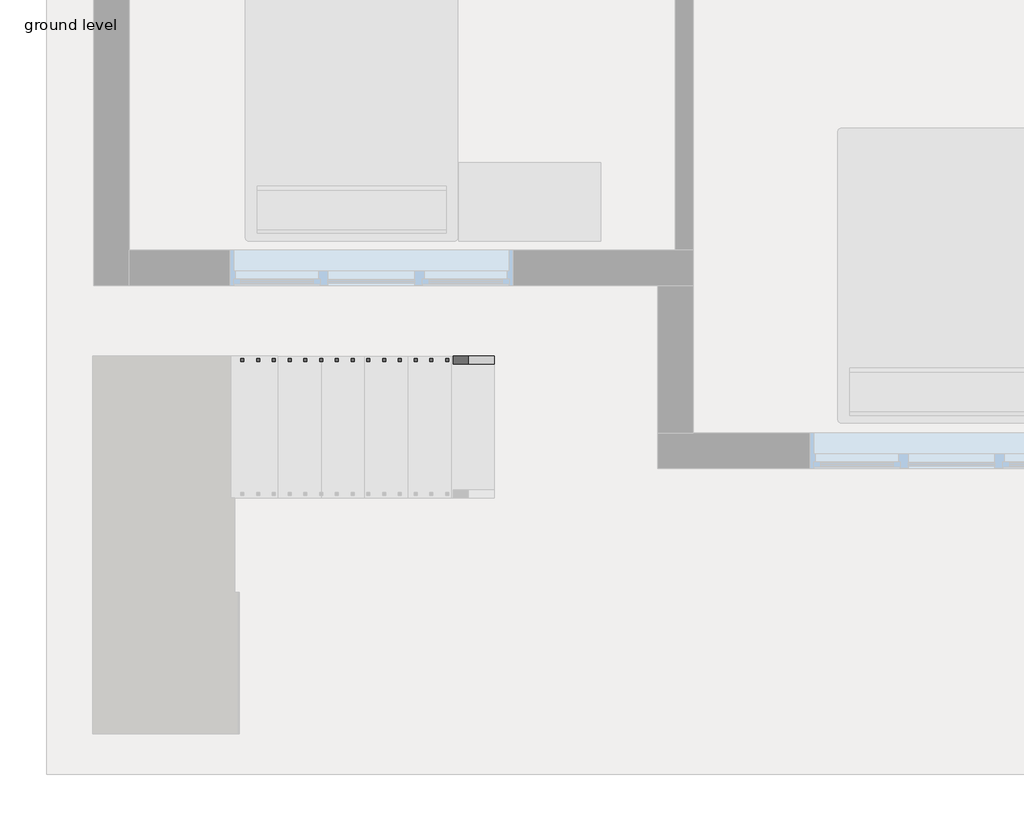
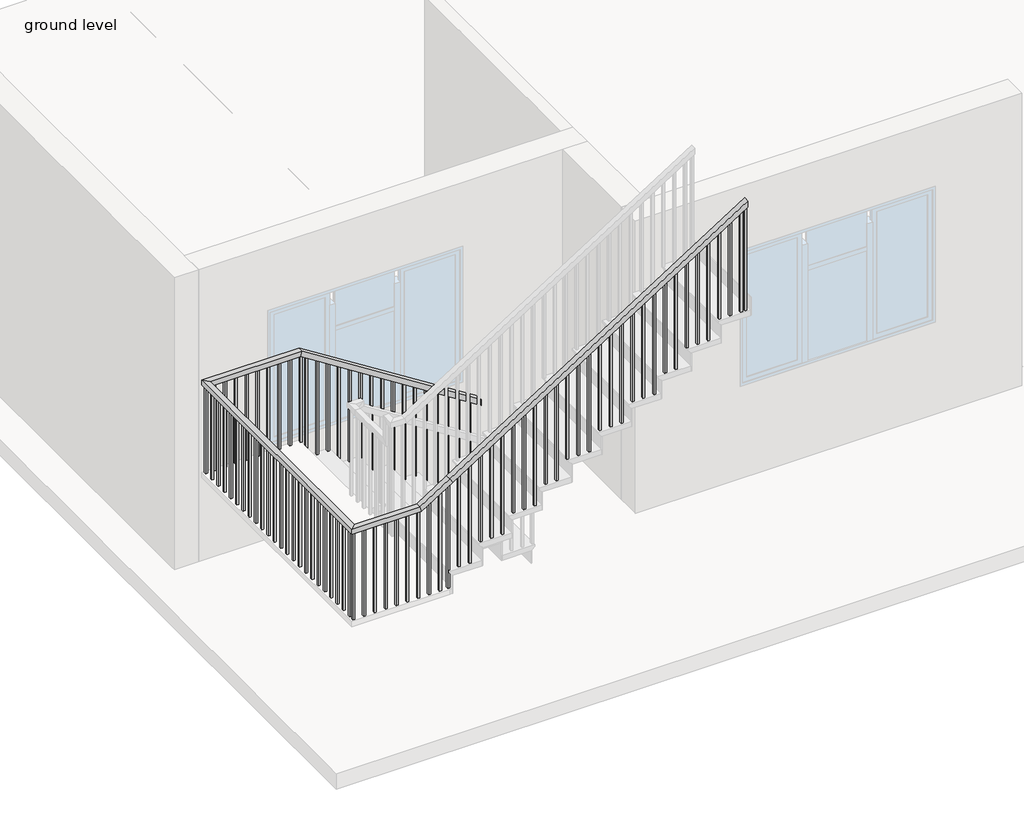
# One storey, part 3 of 4: 1 railing.
"""IFC4 building model written with IfcOpenShell, lengths in millimetres."""

from ifc_helpers import new_model, si_unit, frame, origin, place, context, project, spatial, polyline, outline, extrude, faceted_brep, element, save

model = new_model("IFC4")

# Units and contexts
model_context = context("Model", 3, world=origin())
ifc_project = project(units=[si_unit("LENGTHUNIT", "METRE", prefix="MILLI")], contexts=[model_context])

# Site, building, storey
site = spatial("IfcSite", under=ifc_project)
building = spatial("IfcBuilding", under=site)
storey = spatial("IfcBuildingStorey", under=building, Name="ground level", Elevation=609.6)

# Railing
placement = place(None, origin())
element("IfcRailing", 1, ObjectType="Handrail - Rectangular", at=placement, inside=storey, context=model_context, shape_type="SolidModel", body=[
    faceted_brep([(-6576.0763529, -1102.4338022, 1701.8), (-6576.0763529, -1102.4338022, 1641.586276), (-6576.0763529, -1051.6338022, 1641.586276), (-6576.0763529, -1051.6338022, 1701.8), (-8252.4763529, -1102.4338022, 2768.6), (-8267.2693478, -1102.4338022, 2717.8), (-8267.2693478, -1051.6338022, 2717.8), (-8252.4763529, -1051.6338022, 2768.6), (-9116.0763529, -1102.4338022, 2768.6), (-9116.0763529, -1102.4338022, 2717.8), (-9166.8763529, -1051.6338022, 2717.8), (-9166.8763529, -1051.6338022, 2768.6), (-9116.0763529, -3439.2338022, 2768.6), (-9116.0763529, -3439.2338022, 2717.8), (-9166.8763529, -3490.0338022, 2717.8), (-9166.8763529, -3490.0338022, 2768.6), (-8531.8763529, -3439.2338022, 2768.6), (-8517.083358, -3439.2338022, 2717.8), (-8517.083358, -3490.0338022, 2717.8), (-8531.8763529, -3490.0338022, 2768.6), (-8252.4763529, -3439.2338022, 2946.4), (-8225.2030779, -3439.2338022, 2903.5419964), (-8225.2030779, -3490.0338022, 2903.5419964), (-8252.4763529, -3490.0338022, 2946.4), (-5458.4763529, -3439.2338022, 4724.4), (-5458.4763529, -3490.0338022, 4724.4), (-5458.4763529, -3490.0338022, 4664.186276), (-5458.4763529, -3439.2338022, 4664.186276)], [[[0, 1, 2, 3]], [[1, 0, 4, 5]], [[2, 1, 5, 6]], [[3, 2, 6, 7]], [[0, 3, 7, 4]], [[5, 4, 8, 9]], [[6, 5, 9, 10]], [[7, 6, 10, 11]], [[4, 7, 11, 8]], [[9, 8, 12, 13]], [[10, 9, 13, 14]], [[11, 10, 14, 15]], [[8, 11, 15, 12]], [[13, 12, 16, 17]], [[14, 13, 17, 18]], [[15, 14, 18, 19]], [[12, 15, 19, 16]], [[17, 16, 20, 21]], [[18, 17, 21, 22]], [[19, 18, 22, 23]], [[16, 19, 23, 20]], [[24, 25, 26, 27]], [[21, 20, 24, 27]], [[22, 21, 27, 26]], [[23, 22, 26, 25]], [[20, 23, 25, 24]]]),
    extrude(outline(polyline([(4637.9203669, -5499.7513529), (4625.7976396, -5518.8013529), (3632.2, -5518.8013529), (3632.2, -5499.7513529), (4637.9203669, -5499.7513529)])), frame((0.0, -3474.1588022, 0.0), z_axis=(0.0, 1.0, 0.0), x_axis=(0.0, 0.0, 1.0)), (0.0, 0.0, 1.0), 19.05),
    extrude(outline(polyline([(4573.2658214, -5601.3513529), (4561.1430941, -5620.4013529), (3632.2, -5620.4013529), (3632.2, -5601.3513529), (4573.2658214, -5601.3513529)])), frame((0.0, -3474.1588022, 0.0), z_axis=(0.0, 1.0, 0.0), x_axis=(0.0, 0.0, 1.0)), (0.0, 0.0, 1.0), 19.05),
    extrude(outline(polyline([(4508.611276, -5702.9513529), (4496.4885487, -5722.0013529), (3632.2, -5722.0013529), (3632.2, -5702.9513529), (4508.611276, -5702.9513529)])), frame((0.0, -3474.1588022, 0.0), z_axis=(0.0, 1.0, 0.0), x_axis=(0.0, 0.0, 1.0)), (0.0, 0.0, 1.0), 19.05),
    extrude(outline(polyline([(4443.9567305, -5804.5513529), (4431.8340032, -5823.6013529), (3454.4, -5823.6013529), (3454.4, -5804.5513529), (4443.9567305, -5804.5513529)])), frame((0.0, -3474.1588022, 0.0), z_axis=(0.0, 1.0, 0.0), x_axis=(0.0, 0.0, 1.0)), (0.0, 0.0, 1.0), 19.05),
    extrude(outline(polyline([(4379.3021851, -5906.1513529), (4367.1794578, -5925.2013529), (3454.4, -5925.2013529), (3454.4, -5906.1513529), (4379.3021851, -5906.1513529)])), frame((0.0, -3474.1588022, 0.0), z_axis=(0.0, 1.0, 0.0), x_axis=(0.0, 0.0, 1.0)), (0.0, 0.0, 1.0), 19.05),
    extrude(outline(polyline([(4314.6476396, -6007.7513529), (4302.5249123, -6026.8013529), (3454.4, -6026.8013529), (3454.4, -6007.7513529), (4314.6476396, -6007.7513529)])), frame((0.0, -3474.1588022, 0.0), z_axis=(0.0, 1.0, 0.0), x_axis=(0.0, 0.0, 1.0)), (0.0, 0.0, 1.0), 19.05),
    extrude(outline(polyline([(4249.9930941, -6109.3513529), (4237.8703669, -6128.4013529), (3276.6, -6128.4013529), (3276.6, -6109.3513529), (4249.9930941, -6109.3513529)])), frame((0.0, -3474.1588022, 0.0), z_axis=(0.0, 1.0, 0.0), x_axis=(0.0, 0.0, 1.0)), (0.0, 0.0, 1.0), 19.05),
    extrude(outline(polyline([(4185.3385487, -6210.9513529), (4173.2158214, -6230.0013529), (3276.6, -6230.0013529), (3276.6, -6210.9513529), (4185.3385487, -6210.9513529)])), frame((0.0, -3474.1588022, 0.0), z_axis=(0.0, 1.0, 0.0), x_axis=(0.0, 0.0, 1.0)), (0.0, 0.0, 1.0), 19.05),
    extrude(outline(polyline([(4120.6840032, -6312.5513529), (4108.561276, -6331.6013529), (3098.8, -6331.6013529), (3098.8, -6312.5513529), (4120.6840032, -6312.5513529)])), frame((0.0, -3474.1588022, 0.0), z_axis=(0.0, 1.0, 0.0), x_axis=(0.0, 0.0, 1.0)), (0.0, 0.0, 1.0), 19.05),
    extrude(outline(polyline([(4056.0294578, -6414.1513529), (4043.9067305, -6433.2013529), (3098.8, -6433.2013529), (3098.8, -6414.1513529), (4056.0294578, -6414.1513529)])), frame((0.0, -3474.1588022, 0.0), z_axis=(0.0, 1.0, 0.0), x_axis=(0.0, 0.0, 1.0)), (0.0, 0.0, 1.0), 19.05),
    extrude(outline(polyline([(3991.3749123, -6515.7513529), (3979.2521851, -6534.8013529), (3098.8, -6534.8013529), (3098.8, -6515.7513529), (3991.3749123, -6515.7513529)])), frame((0.0, -3474.1588022, 0.0), z_axis=(0.0, 1.0, 0.0), x_axis=(0.0, 0.0, 1.0)), (0.0, 0.0, 1.0), 19.05),
    extrude(outline(polyline([(3926.7203669, -6617.3513529), (3914.5976396, -6636.4013529), (2921.0, -6636.4013529), (2921.0, -6617.3513529), (3926.7203669, -6617.3513529)])), frame((0.0, -3474.1588022, 0.0), z_axis=(0.0, 1.0, 0.0), x_axis=(0.0, 0.0, 1.0)), (0.0, 0.0, 1.0), 19.05),
    extrude(outline(polyline([(3862.0658214, -6718.9513529), (3849.9430941, -6738.0013529), (2921.0, -6738.0013529), (2921.0, -6718.9513529), (3862.0658214, -6718.9513529)])), frame((0.0, -3474.1588022, 0.0), z_axis=(0.0, 1.0, 0.0), x_axis=(0.0, 0.0, 1.0)), (0.0, 0.0, 1.0), 19.05),
    extrude(outline(polyline([(3797.411276, -6820.5513529), (3785.2885487, -6839.6013529), (2921.0, -6839.6013529), (2921.0, -6820.5513529), (3797.411276, -6820.5513529)])), frame((0.0, -3474.1588022, 0.0), z_axis=(0.0, 1.0, 0.0), x_axis=(0.0, 0.0, 1.0)), (0.0, 0.0, 1.0), 19.05),
    extrude(outline(polyline([(3732.7567305, -6922.1513529), (3720.6340032, -6941.2013529), (2743.2, -6941.2013529), (2743.2, -6922.1513529), (3732.7567305, -6922.1513529)])), frame((0.0, -3474.1588022, 0.0), z_axis=(0.0, 1.0, 0.0), x_axis=(0.0, 0.0, 1.0)), (0.0, 0.0, 1.0), 19.05),
    extrude(outline(polyline([(3668.1021851, -7023.7513529), (3655.9794578, -7042.8013529), (2743.2, -7042.8013529), (2743.2, -7023.7513529), (3668.1021851, -7023.7513529)])), frame((0.0, -3474.1588022, 0.0), z_axis=(0.0, 1.0, 0.0), x_axis=(0.0, 0.0, 1.0)), (0.0, 0.0, 1.0), 19.05),
    extrude(outline(polyline([(3603.4476396, -7125.3513529), (3591.3249123, -7144.4013529), (2743.2, -7144.4013529), (2743.2, -7125.3513529), (3603.4476396, -7125.3513529)])), frame((0.0, -3474.1588022, 0.0), z_axis=(0.0, 1.0, 0.0), x_axis=(0.0, 0.0, 1.0)), (0.0, 0.0, 1.0), 19.05),
    extrude(outline(polyline([(3538.7930941, -7226.9513529), (3526.6703669, -7246.0013529), (2565.4, -7246.0013529), (2565.4, -7226.9513529), (3538.7930941, -7226.9513529)])), frame((0.0, -3474.1588022, 0.0), z_axis=(0.0, 1.0, 0.0), x_axis=(0.0, 0.0, 1.0)), (0.0, 0.0, 1.0), 19.05),
    extrude(outline(polyline([(3474.1385487, -7328.5513529), (3462.0158214, -7347.6013529), (2565.4, -7347.6013529), (2565.4, -7328.5513529), (3474.1385487, -7328.5513529)])), frame((0.0, -3474.1588022, 0.0), z_axis=(0.0, 1.0, 0.0), x_axis=(0.0, 0.0, 1.0)), (0.0, 0.0, 1.0), 19.05),
    extrude(outline(polyline([(3409.4840032, -7430.1513529), (3397.361276, -7449.2013529), (2387.6, -7449.2013529), (2387.6, -7430.1513529), (3409.4840032, -7430.1513529)])), frame((0.0, -3474.1588022, 0.0), z_axis=(0.0, 1.0, 0.0), x_axis=(0.0, 0.0, 1.0)), (0.0, 0.0, 1.0), 19.05),
    extrude(outline(polyline([(3344.8294578, -7531.7513529), (3332.7067305, -7550.8013529), (2387.6, -7550.8013529), (2387.6, -7531.7513529), (3344.8294578, -7531.7513529)])), frame((0.0, -3474.1588022, 0.0), z_axis=(0.0, 1.0, 0.0), x_axis=(0.0, 0.0, 1.0)), (0.0, 0.0, 1.0), 19.05),
    extrude(outline(polyline([(3280.1749123, -7633.3513529), (3268.0521851, -7652.4013529), (2387.6, -7652.4013529), (2387.6, -7633.3513529), (3280.1749123, -7633.3513529)])), frame((0.0, -3474.1588022, 0.0), z_axis=(0.0, 1.0, 0.0), x_axis=(0.0, 0.0, 1.0)), (0.0, 0.0, 1.0), 19.05),
    extrude(outline(polyline([(3215.5203669, -7734.9513529), (3203.3976396, -7754.0013529), (2209.8, -7754.0013529), (2209.8, -7734.9513529), (3215.5203669, -7734.9513529)])), frame((0.0, -3474.1588022, 0.0), z_axis=(0.0, 1.0, 0.0), x_axis=(0.0, 0.0, 1.0)), (0.0, 0.0, 1.0), 19.05),
    extrude(outline(polyline([(3150.8658214, -7836.5513529), (3138.7430941, -7855.6013529), (2209.8, -7855.6013529), (2209.8, -7836.5513529), (3150.8658214, -7836.5513529)])), frame((0.0, -3474.1588022, 0.0), z_axis=(0.0, 1.0, 0.0), x_axis=(0.0, 0.0, 1.0)), (0.0, 0.0, 1.0), 19.05),
    extrude(outline(polyline([(3086.211276, -7938.1513529), (3074.0885487, -7957.2013529), (2209.8, -7957.2013529), (2209.8, -7938.1513529), (3086.211276, -7938.1513529)])), frame((0.0, -3474.1588022, 0.0), z_axis=(0.0, 1.0, 0.0), x_axis=(0.0, 0.0, 1.0)), (0.0, 0.0, 1.0), 19.05),
    extrude(outline(polyline([(3021.5567305, -8039.7513529), (3009.4340032, -8058.8013529), (2032.0, -8058.8013529), (2032.0, -8039.7513529), (3021.5567305, -8039.7513529)])), frame((0.0, -3474.1588022, 0.0), z_axis=(0.0, 1.0, 0.0), x_axis=(0.0, 0.0, 1.0)), (0.0, 0.0, 1.0), 19.05),
    extrude(outline(polyline([(2956.9021851, -8141.3513529), (2944.7794578, -8160.4013529), (2032.0, -8160.4013529), (2032.0, -8141.3513529), (2956.9021851, -8141.3513529)])), frame((0.0, -3474.1588022, 0.0), z_axis=(0.0, 1.0, 0.0), x_axis=(0.0, 0.0, 1.0)), (0.0, 0.0, 1.0), 19.05),
    extrude(outline(polyline([(2843.7567305, -8319.1513529), (2831.6340032, -8338.2013529), (1854.2, -8338.2013529), (1854.2, -8319.1513529), (2843.7567305, -8319.1513529)])), frame((0.0, -3474.1588022, 0.0), z_axis=(0.0, 1.0, 0.0), x_axis=(0.0, 0.0, 1.0)), (0.0, 0.0, 1.0), 19.05),
    extrude(outline(polyline([(2779.1021851, -8420.7513529), (2766.9794578, -8439.8013529), (1854.2, -8439.8013529), (1854.2, -8420.7513529), (2779.1021851, -8420.7513529)])), frame((0.0, -3474.1588022, 0.0), z_axis=(0.0, 1.0, 0.0), x_axis=(0.0, 0.0, 1.0)), (0.0, 0.0, 1.0), 19.05),
    extrude(outline(polyline([(-8541.4013529, -3474.1588022), (-8541.4013529, -3455.1088022), (-8522.3513529, -3455.1088022), (-8522.3513529, -3474.1588022), (-8541.4013529, -3474.1588022)])), frame((0.0, 0.0, 1854.2), z_axis=(0.0, 0.0, 1.0), x_axis=(1.0, 0.0, 0.0)), (0.0, 0.0, 1.0), 863.6),
    extrude(outline(polyline([(-8643.0013529, -3474.1588022), (-8643.0013529, -3455.1088022), (-8623.9513529, -3455.1088022), (-8623.9513529, -3474.1588022), (-8643.0013529, -3474.1588022)])), frame((0.0, 0.0, 1854.2), z_axis=(0.0, 0.0, 1.0), x_axis=(1.0, 0.0, 0.0)), (0.0, 0.0, 1.0), 863.6),
    extrude(outline(polyline([(-8744.6013529, -3474.1588022), (-8744.6013529, -3455.1088022), (-8725.5513529, -3455.1088022), (-8725.5513529, -3474.1588022), (-8744.6013529, -3474.1588022)])), frame((0.0, 0.0, 1854.2), z_axis=(0.0, 0.0, 1.0), x_axis=(1.0, 0.0, 0.0)), (0.0, 0.0, 1.0), 863.6),
    extrude(outline(polyline([(-8846.2013529, -3474.1588022), (-8846.2013529, -3455.1088022), (-8827.1513529, -3455.1088022), (-8827.1513529, -3474.1588022), (-8846.2013529, -3474.1588022)])), frame((0.0, 0.0, 1854.2), z_axis=(0.0, 0.0, 1.0), x_axis=(1.0, 0.0, 0.0)), (0.0, 0.0, 1.0), 863.6),
    extrude(outline(polyline([(-8947.8013529, -3474.1588022), (-8947.8013529, -3455.1088022), (-8928.7513529, -3455.1088022), (-8928.7513529, -3474.1588022), (-8947.8013529, -3474.1588022)])), frame((0.0, 0.0, 1854.2), z_axis=(0.0, 0.0, 1.0), x_axis=(1.0, 0.0, 0.0)), (0.0, 0.0, 1.0), 863.6),
    extrude(outline(polyline([(-9049.4013529, -3474.1588022), (-9049.4013529, -3455.1088022), (-9030.3513529, -3455.1088022), (-9030.3513529, -3474.1588022), (-9049.4013529, -3474.1588022)])), frame((0.0, 0.0, 1854.2), z_axis=(0.0, 0.0, 1.0), x_axis=(1.0, 0.0, 0.0)), (0.0, 0.0, 1.0), 863.6),
    extrude(outline(polyline([(-9151.0013529, -3404.3088022), (-9131.9513529, -3404.3088022), (-9131.9513529, -3423.3588022), (-9151.0013529, -3423.3588022), (-9151.0013529, -3404.3088022)])), frame((0.0, 0.0, 1854.2), z_axis=(0.0, 0.0, 1.0), x_axis=(1.0, 0.0, 0.0)), (0.0, 0.0, 1.0), 863.6),
    extrude(outline(polyline([(-9151.0013529, -3302.7088022), (-9131.9513529, -3302.7088022), (-9131.9513529, -3321.7588022), (-9151.0013529, -3321.7588022), (-9151.0013529, -3302.7088022)])), frame((0.0, 0.0, 1854.2), z_axis=(0.0, 0.0, 1.0), x_axis=(1.0, 0.0, 0.0)), (0.0, 0.0, 1.0), 863.6),
    extrude(outline(polyline([(-9151.0013529, -3201.1088022), (-9131.9513529, -3201.1088022), (-9131.9513529, -3220.1588022), (-9151.0013529, -3220.1588022), (-9151.0013529, -3201.1088022)])), frame((0.0, 0.0, 1854.2), z_axis=(0.0, 0.0, 1.0), x_axis=(1.0, 0.0, 0.0)), (0.0, 0.0, 1.0), 863.6),
    extrude(outline(polyline([(-9151.0013529, -3099.5088022), (-9131.9513529, -3099.5088022), (-9131.9513529, -3118.5588022), (-9151.0013529, -3118.5588022), (-9151.0013529, -3099.5088022)])), frame((0.0, 0.0, 1854.2), z_axis=(0.0, 0.0, 1.0), x_axis=(1.0, 0.0, 0.0)), (0.0, 0.0, 1.0), 863.6),
    extrude(outline(polyline([(-9151.0013529, -2997.9088022), (-9131.9513529, -2997.9088022), (-9131.9513529, -3016.9588022), (-9151.0013529, -3016.9588022), (-9151.0013529, -2997.9088022)])), frame((0.0, 0.0, 1854.2), z_axis=(0.0, 0.0, 1.0), x_axis=(1.0, 0.0, 0.0)), (0.0, 0.0, 1.0), 863.6),
    extrude(outline(polyline([(-9151.0013529, -2896.3088022), (-9131.9513529, -2896.3088022), (-9131.9513529, -2915.3588022), (-9151.0013529, -2915.3588022), (-9151.0013529, -2896.3088022)])), frame((0.0, 0.0, 1854.2), z_axis=(0.0, 0.0, 1.0), x_axis=(1.0, 0.0, 0.0)), (0.0, 0.0, 1.0), 863.6),
    extrude(outline(polyline([(-9151.0013529, -2794.7088022), (-9131.9513529, -2794.7088022), (-9131.9513529, -2813.7588022), (-9151.0013529, -2813.7588022), (-9151.0013529, -2794.7088022)])), frame((0.0, 0.0, 1854.2), z_axis=(0.0, 0.0, 1.0), x_axis=(1.0, 0.0, 0.0)), (0.0, 0.0, 1.0), 863.6),
    extrude(outline(polyline([(-9151.0013529, -2693.1088022), (-9131.9513529, -2693.1088022), (-9131.9513529, -2712.1588022), (-9151.0013529, -2712.1588022), (-9151.0013529, -2693.1088022)])), frame((0.0, 0.0, 1854.2), z_axis=(0.0, 0.0, 1.0), x_axis=(1.0, 0.0, 0.0)), (0.0, 0.0, 1.0), 863.6),
    extrude(outline(polyline([(-9151.0013529, -2591.5088022), (-9131.9513529, -2591.5088022), (-9131.9513529, -2610.5588022), (-9151.0013529, -2610.5588022), (-9151.0013529, -2591.5088022)])), frame((0.0, 0.0, 1854.2), z_axis=(0.0, 0.0, 1.0), x_axis=(1.0, 0.0, 0.0)), (0.0, 0.0, 1.0), 863.6),
    extrude(outline(polyline([(-9151.0013529, -2489.9088022), (-9131.9513529, -2489.9088022), (-9131.9513529, -2508.9588022), (-9151.0013529, -2508.9588022), (-9151.0013529, -2489.9088022)])), frame((0.0, 0.0, 1854.2), z_axis=(0.0, 0.0, 1.0), x_axis=(1.0, 0.0, 0.0)), (0.0, 0.0, 1.0), 863.6),
    extrude(outline(polyline([(-9151.0013529, -2388.3088022), (-9131.9513529, -2388.3088022), (-9131.9513529, -2407.3588022), (-9151.0013529, -2407.3588022), (-9151.0013529, -2388.3088022)])), frame((0.0, 0.0, 1854.2), z_axis=(0.0, 0.0, 1.0), x_axis=(1.0, 0.0, 0.0)), (0.0, 0.0, 1.0), 863.6),
    extrude(outline(polyline([(-9151.0013529, -2286.7088022), (-9131.9513529, -2286.7088022), (-9131.9513529, -2305.7588022), (-9151.0013529, -2305.7588022), (-9151.0013529, -2286.7088022)])), frame((0.0, 0.0, 1854.2), z_axis=(0.0, 0.0, 1.0), x_axis=(1.0, 0.0, 0.0)), (0.0, 0.0, 1.0), 863.6),
    extrude(outline(polyline([(-9151.0013529, -2185.1088022), (-9131.9513529, -2185.1088022), (-9131.9513529, -2204.1588022), (-9151.0013529, -2204.1588022), (-9151.0013529, -2185.1088022)])), frame((0.0, 0.0, 1854.2), z_axis=(0.0, 0.0, 1.0), x_axis=(1.0, 0.0, 0.0)), (0.0, 0.0, 1.0), 863.6),
    extrude(outline(polyline([(-9151.0013529, -2083.5088022), (-9131.9513529, -2083.5088022), (-9131.9513529, -2102.5588022), (-9151.0013529, -2102.5588022), (-9151.0013529, -2083.5088022)])), frame((0.0, 0.0, 1854.2), z_axis=(0.0, 0.0, 1.0), x_axis=(1.0, 0.0, 0.0)), (0.0, 0.0, 1.0), 863.6),
    extrude(outline(polyline([(-9151.0013529, -1981.9088022), (-9131.9513529, -1981.9088022), (-9131.9513529, -2000.9588022), (-9151.0013529, -2000.9588022), (-9151.0013529, -1981.9088022)])), frame((0.0, 0.0, 1854.2), z_axis=(0.0, 0.0, 1.0), x_axis=(1.0, 0.0, 0.0)), (0.0, 0.0, 1.0), 863.6),
    extrude(outline(polyline([(-9151.0013529, -1880.3088022), (-9131.9513529, -1880.3088022), (-9131.9513529, -1899.3588022), (-9151.0013529, -1899.3588022), (-9151.0013529, -1880.3088022)])), frame((0.0, 0.0, 1854.2), z_axis=(0.0, 0.0, 1.0), x_axis=(1.0, 0.0, 0.0)), (0.0, 0.0, 1.0), 863.6),
    extrude(outline(polyline([(-9151.0013529, -1778.7088022), (-9131.9513529, -1778.7088022), (-9131.9513529, -1797.7588022), (-9151.0013529, -1797.7588022), (-9151.0013529, -1778.7088022)])), frame((0.0, 0.0, 1854.2), z_axis=(0.0, 0.0, 1.0), x_axis=(1.0, 0.0, 0.0)), (0.0, 0.0, 1.0), 863.6),
    extrude(outline(polyline([(-9151.0013529, -1677.1088022), (-9131.9513529, -1677.1088022), (-9131.9513529, -1696.1588022), (-9151.0013529, -1696.1588022), (-9151.0013529, -1677.1088022)])), frame((0.0, 0.0, 1854.2), z_axis=(0.0, 0.0, 1.0), x_axis=(1.0, 0.0, 0.0)), (0.0, 0.0, 1.0), 863.6),
    extrude(outline(polyline([(-9151.0013529, -1575.5088022), (-9131.9513529, -1575.5088022), (-9131.9513529, -1594.5588022), (-9151.0013529, -1594.5588022), (-9151.0013529, -1575.5088022)])), frame((0.0, 0.0, 1854.2), z_axis=(0.0, 0.0, 1.0), x_axis=(1.0, 0.0, 0.0)), (0.0, 0.0, 1.0), 863.6),
    extrude(outline(polyline([(-9151.0013529, -1473.9088022), (-9131.9513529, -1473.9088022), (-9131.9513529, -1492.9588022), (-9151.0013529, -1492.9588022), (-9151.0013529, -1473.9088022)])), frame((0.0, 0.0, 1854.2), z_axis=(0.0, 0.0, 1.0), x_axis=(1.0, 0.0, 0.0)), (0.0, 0.0, 1.0), 863.6),
    extrude(outline(polyline([(-9151.0013529, -1372.3088022), (-9131.9513529, -1372.3088022), (-9131.9513529, -1391.3588022), (-9151.0013529, -1391.3588022), (-9151.0013529, -1372.3088022)])), frame((0.0, 0.0, 1854.2), z_axis=(0.0, 0.0, 1.0), x_axis=(1.0, 0.0, 0.0)), (0.0, 0.0, 1.0), 863.6),
    extrude(outline(polyline([(-9151.0013529, -1270.7088022), (-9131.9513529, -1270.7088022), (-9131.9513529, -1289.7588022), (-9151.0013529, -1289.7588022), (-9151.0013529, -1270.7088022)])), frame((0.0, 0.0, 1854.2), z_axis=(0.0, 0.0, 1.0), x_axis=(1.0, 0.0, 0.0)), (0.0, 0.0, 1.0), 863.6),
    extrude(outline(polyline([(-9151.0013529, -1169.1088022), (-9131.9513529, -1169.1088022), (-9131.9513529, -1188.1588022), (-9151.0013529, -1188.1588022), (-9151.0013529, -1169.1088022)])), frame((0.0, 0.0, 1854.2), z_axis=(0.0, 0.0, 1.0), x_axis=(1.0, 0.0, 0.0)), (0.0, 0.0, 1.0), 863.6),
    extrude(outline(polyline([(-9055.7513529, -1067.5088022), (-9055.7513529, -1086.5588022), (-9074.8013529, -1086.5588022), (-9074.8013529, -1067.5088022), (-9055.7513529, -1067.5088022)])), frame((0.0, 0.0, 1854.2), z_axis=(0.0, 0.0, 1.0), x_axis=(1.0, 0.0, 0.0)), (0.0, 0.0, 1.0), 863.6),
    extrude(outline(polyline([(-8954.1513529, -1067.5088022), (-8954.1513529, -1086.5588022), (-8973.2013529, -1086.5588022), (-8973.2013529, -1067.5088022), (-8954.1513529, -1067.5088022)])), frame((0.0, 0.0, 1854.2), z_axis=(0.0, 0.0, 1.0), x_axis=(1.0, 0.0, 0.0)), (0.0, 0.0, 1.0), 863.6),
    extrude(outline(polyline([(-8852.5513529, -1067.5088022), (-8852.5513529, -1086.5588022), (-8871.6013529, -1086.5588022), (-8871.6013529, -1067.5088022), (-8852.5513529, -1067.5088022)])), frame((0.0, 0.0, 1854.2), z_axis=(0.0, 0.0, 1.0), x_axis=(1.0, 0.0, 0.0)), (0.0, 0.0, 1.0), 863.6),
    extrude(outline(polyline([(-8750.9513529, -1067.5088022), (-8750.9513529, -1086.5588022), (-8770.0013529, -1086.5588022), (-8770.0013529, -1067.5088022), (-8750.9513529, -1067.5088022)])), frame((0.0, 0.0, 1854.2), z_axis=(0.0, 0.0, 1.0), x_axis=(1.0, 0.0, 0.0)), (0.0, 0.0, 1.0), 863.6),
    extrude(outline(polyline([(-8649.3513529, -1067.5088022), (-8649.3513529, -1086.5588022), (-8668.4013529, -1086.5588022), (-8668.4013529, -1067.5088022), (-8649.3513529, -1067.5088022)])), frame((0.0, 0.0, 1854.2), z_axis=(0.0, 0.0, 1.0), x_axis=(1.0, 0.0, 0.0)), (0.0, 0.0, 1.0), 863.6),
    extrude(outline(polyline([(-8547.7513529, -1067.5088022), (-8547.7513529, -1086.5588022), (-8566.8013529, -1086.5588022), (-8566.8013529, -1067.5088022), (-8547.7513529, -1067.5088022)])), frame((0.0, 0.0, 1854.2), z_axis=(0.0, 0.0, 1.0), x_axis=(1.0, 0.0, 0.0)), (0.0, 0.0, 1.0), 863.6),
    extrude(outline(polyline([(-8446.1513529, -1067.5088022), (-8446.1513529, -1086.5588022), (-8465.2013529, -1086.5588022), (-8465.2013529, -1067.5088022), (-8446.1513529, -1067.5088022)])), frame((0.0, 0.0, 1854.2), z_axis=(0.0, 0.0, 1.0), x_axis=(1.0, 0.0, 0.0)), (0.0, 0.0, 1.0), 863.6),
    extrude(outline(polyline([(-8344.5513529, -1067.5088022), (-8344.5513529, -1086.5588022), (-8363.6013529, -1086.5588022), (-8363.6013529, -1067.5088022), (-8344.5513529, -1067.5088022)])), frame((0.0, 0.0, 1854.2), z_axis=(0.0, 0.0, 1.0), x_axis=(1.0, 0.0, 0.0)), (0.0, 0.0, 1.0), 863.6),
    extrude(outline(polyline([(2669.9976396, -8192.1513529), (2682.1203669, -8211.2013529), (1676.4, -8211.2013529), (1676.4, -8192.1513529), (2669.9976396, -8192.1513529)])), frame((0.0, -1086.5588022, 0.0), z_axis=(0.0, 1.0, 0.0), x_axis=(0.0, 0.0, 1.0)), (0.0, 0.0, 1.0), 19.05),
    extrude(outline(polyline([(2605.3430941, -8090.5513529), (2617.4658214, -8109.6013529), (1676.4, -8109.6013529), (1676.4, -8090.5513529), (2605.3430941, -8090.5513529)])), frame((0.0, -1086.5588022, 0.0), z_axis=(0.0, 1.0, 0.0), x_axis=(0.0, 0.0, 1.0)), (0.0, 0.0, 1.0), 19.05),
    extrude(outline(polyline([(2540.6885487, -7988.9513529), (2552.811276, -8008.0013529), (1676.4, -8008.0013529), (1676.4, -7988.9513529), (2540.6885487, -7988.9513529)])), frame((0.0, -1086.5588022, 0.0), z_axis=(0.0, 1.0, 0.0), x_axis=(0.0, 0.0, 1.0)), (0.0, 0.0, 1.0), 19.05),
    extrude(outline(polyline([(2476.0340032, -7887.3513529), (2488.1567305, -7906.4013529), (1498.6, -7906.4013529), (1498.6, -7887.3513529), (2476.0340032, -7887.3513529)])), frame((0.0, -1086.5588022, 0.0), z_axis=(0.0, 1.0, 0.0), x_axis=(0.0, 0.0, 1.0)), (0.0, 0.0, 1.0), 19.05),
    extrude(outline(polyline([(2411.3794578, -7785.7513529), (2423.5021851, -7804.8013529), (1498.6, -7804.8013529), (1498.6, -7785.7513529), (2411.3794578, -7785.7513529)])), frame((0.0, -1086.5588022, 0.0), z_axis=(0.0, 1.0, 0.0), x_axis=(0.0, 0.0, 1.0)), (0.0, 0.0, 1.0), 19.05),
    extrude(outline(polyline([(2346.7249123, -7684.1513529), (2358.8476396, -7703.2013529), (1498.6, -7703.2013529), (1498.6, -7684.1513529), (2346.7249123, -7684.1513529)])), frame((0.0, -1086.5588022, 0.0), z_axis=(0.0, 1.0, 0.0), x_axis=(0.0, 0.0, 1.0)), (0.0, 0.0, 1.0), 19.05),
    extrude(outline(polyline([(2282.0703669, -7582.5513529), (2294.1930941, -7601.6013529), (1320.8, -7601.6013529), (1320.8, -7582.5513529), (2282.0703669, -7582.5513529)])), frame((0.0, -1086.5588022, 0.0), z_axis=(0.0, 1.0, 0.0), x_axis=(0.0, 0.0, 1.0)), (0.0, 0.0, 1.0), 19.05),
    extrude(outline(polyline([(2217.4158214, -7480.9513529), (2229.5385487, -7500.0013529), (1320.8, -7500.0013529), (1320.8, -7480.9513529), (2217.4158214, -7480.9513529)])), frame((0.0, -1086.5588022, 0.0), z_axis=(0.0, 1.0, 0.0), x_axis=(0.0, 0.0, 1.0)), (0.0, 0.0, 1.0), 19.05),
    extrude(outline(polyline([(2152.761276, -7379.3513529), (2164.8840032, -7398.4013529), (1143.0, -7398.4013529), (1143.0, -7379.3513529), (2152.761276, -7379.3513529)])), frame((0.0, -1086.5588022, 0.0), z_axis=(0.0, 1.0, 0.0), x_axis=(0.0, 0.0, 1.0)), (0.0, 0.0, 1.0), 19.05),
    extrude(outline(polyline([(2088.1067305, -7277.7513529), (2100.2294578, -7296.8013529), (1143.0, -7296.8013529), (1143.0, -7277.7513529), (2088.1067305, -7277.7513529)])), frame((0.0, -1086.5588022, 0.0), z_axis=(0.0, 1.0, 0.0), x_axis=(0.0, 0.0, 1.0)), (0.0, 0.0, 1.0), 19.05),
    extrude(outline(polyline([(2023.4521851, -7176.1513529), (2035.5749123, -7195.2013529), (1143.0, -7195.2013529), (1143.0, -7176.1513529), (2023.4521851, -7176.1513529)])), frame((0.0, -1086.5588022, 0.0), z_axis=(0.0, 1.0, 0.0), x_axis=(0.0, 0.0, 1.0)), (0.0, 0.0, 1.0), 19.05),
    extrude(outline(polyline([(1958.7976396, -7074.5513529), (1970.9203669, -7093.6013529), (965.2, -7093.6013529), (965.2, -7074.5513529), (1958.7976396, -7074.5513529)])), frame((0.0, -1086.5588022, 0.0), z_axis=(0.0, 1.0, 0.0), x_axis=(0.0, 0.0, 1.0)), (0.0, 0.0, 1.0), 19.05),
    extrude(outline(polyline([(1894.1430941, -6972.9513529), (1906.2658214, -6992.0013529), (965.2, -6992.0013529), (965.2, -6972.9513529), (1894.1430941, -6972.9513529)])), frame((0.0, -1086.5588022, 0.0), z_axis=(0.0, 1.0, 0.0), x_axis=(0.0, 0.0, 1.0)), (0.0, 0.0, 1.0), 19.05),
    extrude(outline(polyline([(1829.4885487, -6871.3513529), (1841.611276, -6890.4013529), (965.2, -6890.4013529), (965.2, -6871.3513529), (1829.4885487, -6871.3513529)])), frame((0.0, -1086.5588022, 0.0), z_axis=(0.0, 1.0, 0.0), x_axis=(0.0, 0.0, 1.0)), (0.0, 0.0, 1.0), 19.05),
    extrude(outline(polyline([(1764.8340032, -6769.7513529), (1776.9567305, -6788.8013529), (787.4, -6788.8013529), (787.4, -6769.7513529), (1764.8340032, -6769.7513529)])), frame((0.0, -1086.5588022, 0.0), z_axis=(0.0, 1.0, 0.0), x_axis=(0.0, 0.0, 1.0)), (0.0, 0.0, 1.0), 19.05),
    extrude(outline(polyline([(1700.1794578, -6668.1513529), (1712.3021851, -6687.2013529), (787.4, -6687.2013529), (787.4, -6668.1513529), (1700.1794578, -6668.1513529)])), frame((0.0, -1086.5588022, 0.0), z_axis=(0.0, 1.0, 0.0), x_axis=(0.0, 0.0, 1.0)), (0.0, 0.0, 1.0), 19.05),
    extrude(outline(polyline([(2892.2476396, -8242.9513529), (2880.1249123, -8262.0013529), (1854.2, -8262.0013529), (1854.2, -8242.9513529), (2892.2476396, -8242.9513529)])), frame((0.0, -3474.1588022, 0.0), z_axis=(0.0, 1.0, 0.0), x_axis=(0.0, 0.0, 1.0)), (0.0, 0.0, 1.0), 19.05),
    extrude(outline(polyline([(-9151.0013529, -3455.1088022), (-9131.9513529, -3455.1088022), (-9131.9513529, -3474.1588022), (-9151.0013529, -3474.1588022), (-9151.0013529, -3455.1088022)])), frame((0.0, 0.0, 1854.2), z_axis=(0.0, 0.0, 1.0), x_axis=(1.0, 0.0, 0.0)), (0.0, 0.0, 1.0), 863.6),
    extrude(outline(polyline([(-9131.9513529, -1067.5088022), (-9131.9513529, -1086.5588022), (-9151.0013529, -1086.5588022), (-9151.0013529, -1067.5088022), (-9131.9513529, -1067.5088022)])), frame((0.0, 0.0, 1854.2), z_axis=(0.0, 0.0, 1.0), x_axis=(1.0, 0.0, 0.0)), (0.0, 0.0, 1.0), 863.6),
    extrude(outline(polyline([(2702.3249123, -8242.9513529), (2714.4476396, -8262.0013529), (1854.2, -8262.0013529), (1854.2, -8242.9513529), (2702.3249123, -8242.9513529)])), frame((0.0, -1086.5588022, 0.0), z_axis=(0.0, 1.0, 0.0), x_axis=(0.0, 0.0, 1.0)), (0.0, 0.0, 1.0), 19.05),
    extrude(outline(polyline([(4664.186276, -5458.4763529), (4652.0635487, -5477.5263529), (3632.2, -5477.5263529), (3632.2, -5458.4763529), (4664.186276, -5458.4763529)])), frame((0.0, -3474.1588022, 0.0), z_axis=(0.0, 1.0, 0.0), x_axis=(0.0, 0.0, 1.0)), (0.0, 0.0, 1.0), 19.05),
    extrude(outline(polyline([(1641.586276, -6576.0763529), (1653.7090032, -6595.1263529), (787.4, -6595.1263529), (787.4, -6576.0763529), (1641.586276, -6576.0763529)])), frame((0.0, -1086.5588022, 0.0), z_axis=(0.0, 1.0, 0.0), x_axis=(0.0, 0.0, 1.0)), (0.0, 0.0, 1.0), 19.05),
])

save(model, "model.ifc")

# Revit data of these elements
# Type "Handrail - Rectangular"
#   Assembly Code = "C2010400"
#   built-in parameter 1008612 = 0.0416667 (stored number, unit not read)
#   built-in parameter 1008611 = 0.0416667 (stored number, unit not read)
#   built-in parameter 1008609 = 0.333333 (stored number, unit not read)
#   built-in parameter 1008604 = 0.166667 (stored number, unit not read)
#   built-in parameter 1008603 = 0.166667 (stored number, unit not read)
#   Railing Height = 3' - 0"
#   built-in parameter 1008630 = 2
#   built-in parameter 1008610 = 2
#   built-in parameter 1008618 = Baluster - Square : 3/4"
# Element 1 (IfcRailing, "Handrail - Rectangular")
#   Phase Created = New Construction
